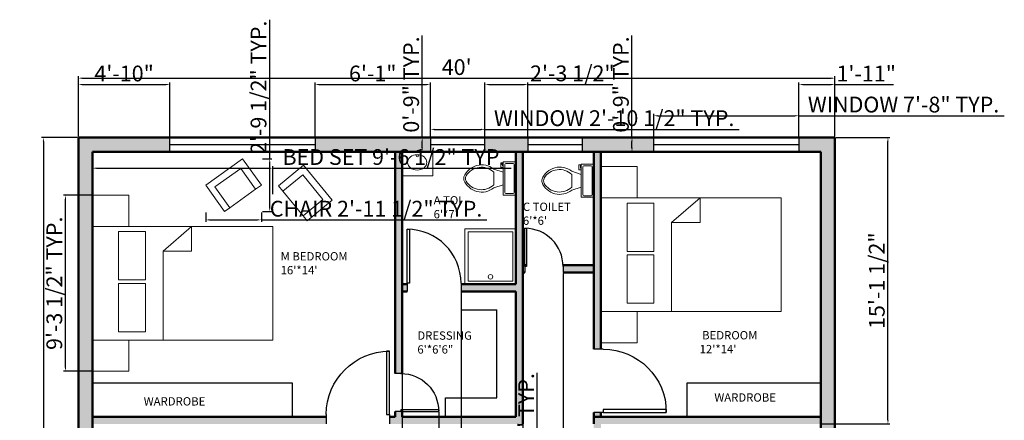
# Model space of a CAD drawing. Units: inches. Extents: x 772 to 1415, y 1573 to 2261.
# Tile 4 of 4: x 790 to 1415, y 2007 to 2261. Entities that reach past the tile are written whole.
import ezdxf

# ---------------------------------------------------------------- set-up
doc = ezdxf.new("R2010")
doc.units = ezdxf.units.IN
for name, color, linetype, lineweight in [('A-ANNO-DIMS', 2, 'Continuous', 18), ('A-ANNO-TEXT', 10, 'Continuous', 25), ('A-AREA-IDEN', 10, 'Continuous', 25), ('A-FLOR-FIXT', 9, 'Continuous', 18), ('A-FURN-FIXD', 210, 'Continuous', 25), ('A-WALL-PATT', 140, 'Continuous', 13), ('DOOR', 52, 'Continuous', 25), ('FUR', 210, 'Continuous', 18), ('WALL', 7, 'Continuous', 50), ('WINDOW', 80, 'Continuous', 25)]:
    doc.layers.add(name, color=color, linetype=linetype, lineweight=lineweight)
doc.styles.get("Standard").update_dxf_attribs({"font": 'arial.ttf'})
doc.dimstyles.new('ISO-25', dxfattribs={"dimtxt": 10, "dimasz": 2.5, "dimexe": 1.25, "dimexo": 0.625, "dimtad": 1, "dimdec": 0, "dimlunit": 4, "dimtxsty": 'Standard', "dimcen": 2.5, "dimadec": 0, "dimazin": 0, "dimtfac": 1, "dimtdec": 0, "dimtmove": 0, "dimatfit": 3, "dimfxl": 1, "dimarcsym": 0})

# ---------------------------------------------------------------- blocks, each defined once
blk = doc.blocks.new('*U2')
for p, q in [((0, 0), (0, -6)), ((40, 0), (40, -6))]:
    blk.add_line(p, q)
blk.add_lwpolyline([(0, 0), (0, 40), (1.75, 40), (1.75, 0)], close=True)
blk.add_arc((0, 0), 40, 0, 90)
blk = doc.blocks.new('*U4')
for p, q in [((9.5, -6), (9.5, -2)), ((-10, -8.5), (-8, -8.5)), ((-10, -9.5), (-10, -8.5)), ((-7, -9.5), (-10, -9.5)), ((-8, -8.5), (-8, -8)), ((-7, -8), (-7, -9.5)), ((-4, -8), (-6, -14)), ((4, -8), (6, -14)), ((4, -14), (-4, -14))]:
    blk.add_line(p, q)
blk.add_lwpolyline([(10.5, -8), (10.5, 0), (-10.5, 0), (-10.5, -8)], close=True)
for points in [[(-9.5, -2), (-9.5, -6)], [(8.5, -1), (-8.5, -1)], [(-8.5, -7), (8.5, -7)]]:
    blk.add_lwpolyline(points)
for centre, radius, start, end in [((-8.62, -1.88), 0.884, 81.8699, 188.1301), ((-8.62, -6.12), 0.884, 171.8699, 278.1301), ((8.62, -1.88), 0.884, 351.8699, 98.1301), ((8.62, -6.12), 0.884, 261.8699, 8.1301), ((3.52, -21.58), 12.17, 141.46911, 247.97143), ((4.2, -21.82), 11.33, 136.36773, 238.94682), ((-3.52, -21.58), 12.17, 292.02843, 38.53071), ((-4.2, -21.82), 11.33, 301.05301, 43.63209), ((0, -27.88), 4, 245.73182, 294.26817), ((0, -29), 4, 254.86053, 285.13947)]:
    blk.add_arc(centre, radius, start, end)
blk = doc.blocks.new('*D9')
at = {"layer": 'A-ANNO-DIMS', "color": 0, "lineweight": -2, "transparency": 16777216}
for p, q in [((827.65, 2186.61), (827.65, 2224.87)), ((1307.65, 2186.61), (1307.65, 2224.87)), ((830.15, 2223.62), (1305.15, 2223.62))]:
    blk.add_line(p, q, dxfattribs=at)
at = {"layer": 'A-ANNO-DIMS', "color": 0, "transparency": 16777216}
for points in [[(830.15, 2224.04), (830.15, 2223.21), (827.65, 2223.62)], [(1305.15, 2224.04), (1305.15, 2223.21), (1307.65, 2223.62)]]:
    blk.add_solid(points, dxfattribs=at)
at = {"layer": 'Defpoints', "color": 0, "transparency": 16777216}
for p in [(1307.65, 2223.62), (827.65, 2185.98), (1307.65, 2185.98)]:
    blk.add_point(p, dxfattribs=at)
at = {"layer": 'A-ANNO-DIMS', "color": 0, "transparency": 16777216, "insert": (1067.65, 2229.36), "char_height": 10, "attachment_point": 5}
blk.add_mtext("40'", dxfattribs=at)
blk = doc.blocks.new('*D10')
at = {"layer": 'A-ANNO-DIMS', "color": 0, "lineweight": -2, "transparency": 16777216}
for p, q in [((827.03, 2185.98), (804.2, 2185.98)), ((805.45, 2183.48), (805.45, 1648.48)), ((827.03, 1645.98), (804.2, 1645.98))]:
    blk.add_line(p, q, dxfattribs=at)
at = {"layer": 'A-ANNO-DIMS', "color": 0, "transparency": 16777216}
for points in [[(805.04, 2183.48), (805.87, 2183.48), (805.45, 2185.98)], [(805.04, 1648.48), (805.87, 1648.48), (805.45, 1645.98)]]:
    blk.add_solid(points, dxfattribs=at)
at = {"layer": 'Defpoints', "color": 0, "transparency": 16777216}
for p in [(827.65, 2185.98), (805.45, 1645.98), (827.65, 1645.98)]:
    blk.add_point(p, dxfattribs=at)
at = {"layer": 'A-ANNO-DIMS', "color": 0, "transparency": 16777216, "insert": (799.74, 1915.98), "char_height": 10, "attachment_point": 5, "rotation": 90}
blk.add_mtext("45'", dxfattribs=at)
blk = doc.blocks.new('BED-DOUBLE-WITH-NIGHTSTANDS')
for p, q in [((62.88, 91.88), (44.81, 76.26)), ((62.88, 76.26), (62.88, 91.88)), ((44.81, 19.73), (44.81, 76.26)), ((44.81, 76.26), (62.88, 76.26))]:
    blk.add_line(p, q)
for points in [[(0, 91.88), (23.11, 91.88), (23.11, 111.61), (0, 111.61)], [(0, 19.73), (114.34, 19.73), (114.34, 91.88), (0, 91.88)], [(16.57, 57.89), (33.66, 57.89), (33.66, 88.54), (16.57, 88.54)], [(16.57, 25.11), (33.66, 25.11), (33.66, 55.76), (16.57, 55.76)], [(0, 0), (23.11, 0), (23.11, 19.73), (0, 19.73)]]:
    blk.add_lwpolyline(points, close=True)
blk = doc.blocks.new('CHAIR-BEDROOM')
for p, q in [((0, 16.64), (23.37, 33.43)), ((23.37, 33.43), (35.32, 16.78)), ((11.95, 0), (0, 16.64)), ((35.32, 16.78), (31.69, 14.18)), ((15.31, 2.41), (11.95, 0))]:
    blk.add_line(p, q)
blk.add_lwpolyline([(15.31, 2.41), (31.69, 14.18), (22.24, 27.34), (5.85, 15.57)], close=True)
blk = doc.blocks.new('WIN-92IN')
blk.add_line((0, 4.5), (92.1, 4.5))
blk.add_lwpolyline([(0, 9), (92.1, 9), (92.1, 0), (0, 0)], close=True)
blk = doc.blocks.new('WIN-35IN')
blk.add_line((0, 4.5), (34.63, 4.5))
blk.add_lwpolyline([(0, 0), (34.63, 0), (34.63, 9), (0, 9)], close=True)
blk = doc.blocks.new('*D21')
at = {"layer": 'A-ANNO-DIMS', "color": 0, "lineweight": -2, "transparency": 16777216}
for p, q in [((836.65, 2150.03), (836.65, 2167.81)), ((950.99, 2150.03), (950.99, 2167.81)), ((839.15, 2166.56), (948.49, 2166.56)), ((950.99, 2166.56), (1102.21, 2166.56))]:
    blk.add_line(p, q, dxfattribs=at)
at = {"layer": 'A-ANNO-DIMS', "color": 0, "transparency": 16777216}
for points in [[(839.15, 2166.97), (839.15, 2166.14), (836.65, 2166.56)], [(948.49, 2166.97), (948.49, 2166.14), (950.99, 2166.56)]]:
    blk.add_solid(points, dxfattribs=at)
at = {"layer": 'Defpoints', "color": 0, "transparency": 16777216}
for p in [(950.99, 2166.56), (836.65, 2149.41), (950.99, 2149.41)]:
    blk.add_point(p, dxfattribs=at)
at = {"layer": 'A-ANNO-DIMS', "color": 0, "transparency": 16777216, "insert": (1027.85, 2172.35), "char_height": 10, "attachment_point": 5}
blk.add_mtext('BED SET 9\'-6 1/2" TYP.', dxfattribs=at)
blk = doc.blocks.new('*D22')
at = {"layer": 'A-ANNO-DIMS', "color": 0, "lineweight": -2, "transparency": 16777216}
for p, q in [((836.03, 2149.41), (818.25, 2149.41)), ((819.5, 2040.29), (819.5, 2146.91)), ((836.03, 2037.79), (818.25, 2037.79))]:
    blk.add_line(p, q, dxfattribs=at)
at = {"layer": 'A-ANNO-DIMS', "color": 0, "transparency": 16777216}
for points in [[(819.08, 2146.91), (819.92, 2146.91), (819.5, 2149.41)], [(819.08, 2040.29), (819.92, 2040.29), (819.5, 2037.79)]]:
    blk.add_solid(points, dxfattribs=at)
at = {"layer": 'Defpoints', "color": 0, "transparency": 16777216}
for p in [(819.5, 2149.41), (836.65, 2149.41), (836.65, 2037.79)]:
    blk.add_point(p, dxfattribs=at)
at = {"layer": 'A-ANNO-DIMS', "color": 0, "transparency": 16777216, "insert": (813.7, 2093.6), "char_height": 10, "attachment_point": 5, "rotation": 90}
blk.add_mtext('9\'-3 1/2" TYP.', dxfattribs=at)
blk = doc.blocks.new('*D23')
at = {"layer": 'A-ANNO-DIMS', "color": 0, "lineweight": -2, "transparency": 16777216}
for p, q in [((908.44, 2138.46), (908.44, 2132.54)), ((943.76, 2138.46), (943.76, 2132.54)), ((910.94, 2133.79), (941.26, 2133.79)), ((943.76, 2133.79), (1086.77, 2133.79))]:
    blk.add_line(p, q, dxfattribs=at)
at = {"layer": 'A-ANNO-DIMS', "color": 0, "transparency": 16777216}
for points in [[(910.94, 2134.21), (910.94, 2133.37), (908.44, 2133.79)], [(941.26, 2134.21), (941.26, 2133.37), (943.76, 2133.79)]]:
    blk.add_solid(points, dxfattribs=at)
at = {"layer": 'Defpoints', "color": 0, "transparency": 16777216}
for p in [(908.44, 2139.09), (943.76, 2139.09), (943.76, 2133.79)]:
    blk.add_point(p, dxfattribs=at)
at = {"layer": 'A-ANNO-DIMS', "color": 0, "transparency": 16777216, "insert": (1016.52, 2139.58), "char_height": 10, "attachment_point": 5}
blk.add_mtext('CHAIR 2\'-11 1/2" TYP.', dxfattribs=at)
blk = doc.blocks.new('*D24')
at = {"layer": 'A-ANNO-DIMS', "color": 0, "lineweight": -2, "transparency": 16777216}
for p, q in [((949.06, 2172.52), (949.06, 2260.69)), ((944.39, 2172.52), (950.31, 2172.52)), ((949.06, 2141.59), (949.06, 2170.02)), ((944.39, 2139.09), (950.31, 2139.09))]:
    blk.add_line(p, q, dxfattribs=at)
at = {"layer": 'A-ANNO-DIMS', "color": 0, "transparency": 16777216}
for points in [[(948.64, 2170.02), (949.48, 2170.02), (949.06, 2172.52)], [(948.64, 2141.59), (949.48, 2141.59), (949.06, 2139.09)]]:
    blk.add_solid(points, dxfattribs=at)
at = {"layer": 'Defpoints', "color": 0, "transparency": 16777216}
for p in [(943.76, 2172.52), (949.06, 2172.52), (943.76, 2139.09)]:
    blk.add_point(p, dxfattribs=at)
at = {"layer": 'A-ANNO-DIMS', "color": 0, "transparency": 16777216, "insert": (943.27, 2217.85), "char_height": 10, "attachment_point": 5, "rotation": 90}
blk.add_mtext('2\'-9 1/2" TYP.', dxfattribs=at)
blk = doc.blocks.new('*D30')
at = {"layer": 'A-ANNO-DIMS', "color": 0, "lineweight": -2, "transparency": 16777216}
for p, q in [((1118.67, 1965.32), (1118.67, 2036.85)), ((1107.43, 1965.32), (1119.92, 1965.32)), ((1118.67, 1944.62), (1118.67, 1962.82)), ((1107.43, 1942.12), (1119.92, 1942.12))]:
    blk.add_line(p, q, dxfattribs=at)
at = {"layer": 'A-ANNO-DIMS', "color": 0, "transparency": 16777216}
for points in [[(1118.25, 1962.82), (1119.09, 1962.82), (1118.67, 1965.32)], [(1118.25, 1944.62), (1119.09, 1944.62), (1118.67, 1942.12)]]:
    blk.add_solid(points, dxfattribs=at)
at = {"layer": 'Defpoints', "color": 0, "transparency": 16777216}
for p in [(1106.81, 1965.32), (1118.67, 1965.32), (1106.81, 1942.12)]:
    blk.add_point(p, dxfattribs=at)
at = {"layer": 'A-ANNO-DIMS', "color": 0, "transparency": 16777216, "insert": (1113.02, 2002.34), "char_height": 10, "attachment_point": 5, "rotation": 90}
blk.add_mtext('1\'-11" TYP.', dxfattribs=at)
blk = doc.blocks.new('*D31')
at = {"layer": 'A-ANNO-DIMS', "color": 0, "lineweight": -2, "transparency": 16777216}
for p, q in [((1192.68, 2186.61), (1192.68, 2201.05)), ((1195.18, 2199.8), (1282.28, 2199.8)), ((1284.78, 2186.61), (1284.78, 2201.05)), ((1284.78, 2199.8), (1415.07, 2199.8))]:
    blk.add_line(p, q, dxfattribs=at)
at = {"layer": 'A-ANNO-DIMS', "color": 0, "transparency": 16777216}
for points in [[(1195.18, 2200.21), (1195.18, 2199.38), (1192.68, 2199.8)], [(1282.28, 2200.21), (1282.28, 2199.38), (1284.78, 2199.8)]]:
    blk.add_solid(points, dxfattribs=at)
at = {"layer": 'Defpoints', "color": 0, "transparency": 16777216}
for p in [(1284.78, 2199.8), (1192.68, 2185.98), (1284.78, 2185.98)]:
    blk.add_point(p, dxfattribs=at)
at = {"layer": 'A-ANNO-DIMS', "color": 0, "transparency": 16777216, "insert": (1351.17, 2205.6), "char_height": 10, "attachment_point": 5}
blk.add_mtext('WINDOW 7\'-8" TYP.', dxfattribs=at)
blk = doc.blocks.new('*D32')
at = {"layer": 'A-ANNO-DIMS', "color": 0, "lineweight": -2, "transparency": 16777216}
for p, q in [((1178.87, 2185.98), (1178.87, 2250.69)), ((1192.06, 2185.98), (1177.62, 2185.98)), ((1178.87, 2179.48), (1178.87, 2183.48)), ((1192.06, 2176.98), (1177.62, 2176.98))]:
    blk.add_line(p, q, dxfattribs=at)
at = {"layer": 'A-ANNO-DIMS', "color": 0, "transparency": 16777216}
for points in [[(1178.45, 2183.48), (1179.28, 2183.48), (1178.87, 2185.98)], [(1178.45, 2179.48), (1179.28, 2179.48), (1178.87, 2176.98)]]:
    blk.add_solid(points, dxfattribs=at)
at = {"layer": 'Defpoints', "color": 0, "transparency": 16777216}
for p in [(1178.87, 2185.98), (1192.68, 2185.98), (1192.68, 2176.98)]:
    blk.add_point(p, dxfattribs=at)
at = {"layer": 'A-ANNO-DIMS', "color": 0, "transparency": 16777216, "insert": (1173.13, 2219.59), "char_height": 10, "attachment_point": 5, "rotation": 90}
blk.add_mtext('0\'-9" TYP.', dxfattribs=at)
blk = doc.blocks.new('*D33')
at = {"layer": 'A-ANNO-DIMS', "color": 0, "lineweight": -2, "transparency": 16777216}
for p, q in [((1050.98, 2186.61), (1050.98, 2192.43)), ((1053.48, 2191.18), (1083.11, 2191.18)), ((1085.61, 2186.61), (1085.61, 2192.43)), ((1085.61, 2191.18), (1246.97, 2191.18))]:
    blk.add_line(p, q, dxfattribs=at)
at = {"layer": 'A-ANNO-DIMS', "color": 0, "transparency": 16777216}
for points in [[(1053.48, 2191.59), (1053.48, 2190.76), (1050.98, 2191.18)], [(1083.11, 2191.59), (1083.11, 2190.76), (1085.61, 2191.18)]]:
    blk.add_solid(points, dxfattribs=at)
at = {"layer": 'Defpoints', "color": 0, "transparency": 16777216}
for p in [(1085.61, 2191.18), (1050.98, 2185.98), (1085.61, 2185.98)]:
    blk.add_point(p, dxfattribs=at)
at = {"layer": 'A-ANNO-DIMS', "color": 0, "transparency": 16777216, "insert": (1167.54, 2196.98), "char_height": 10, "attachment_point": 5}
blk.add_mtext('WINDOW 2\'-10 1/2" TYP.', dxfattribs=at)
blk = doc.blocks.new('*D34')
at = {"layer": 'A-ANNO-DIMS', "color": 0, "lineweight": -2, "transparency": 16777216}
for p, q in [((1045.79, 2185.98), (1045.79, 2250.69)), ((1050.36, 2185.98), (1044.54, 2185.98)), ((1045.79, 2179.48), (1045.79, 2183.48)), ((1050.36, 2176.98), (1044.54, 2176.98))]:
    blk.add_line(p, q, dxfattribs=at)
at = {"layer": 'A-ANNO-DIMS', "color": 0, "transparency": 16777216}
for points in [[(1045.37, 2183.48), (1046.2, 2183.48), (1045.79, 2185.98)], [(1045.37, 2179.48), (1046.2, 2179.48), (1045.79, 2176.98)]]:
    blk.add_solid(points, dxfattribs=at)
at = {"layer": 'Defpoints', "color": 0, "transparency": 16777216}
for p in [(1045.79, 2185.98), (1050.98, 2185.98), (1050.98, 2176.98)]:
    blk.add_point(p, dxfattribs=at)
at = {"layer": 'A-ANNO-DIMS', "color": 0, "transparency": 16777216, "insert": (1040.05, 2219.59), "char_height": 10, "attachment_point": 5, "rotation": 90}
blk.add_mtext('0\'-9" TYP.', dxfattribs=at)
blk = doc.blocks.new('*D47')
at = {"layer": 'A-ANNO-DIMS', "color": 0, "lineweight": -2, "transparency": 16777216}
for p, q in [((1308.28, 2185.98), (1342.5, 2185.98)), ((1341.25, 2006.98), (1341.25, 2183.48)), ((1299.28, 2004.48), (1342.5, 2004.48))]:
    blk.add_line(p, q, dxfattribs=at)
at = {"layer": 'A-ANNO-DIMS', "color": 0, "transparency": 16777216}
for points in [[(1340.83, 2183.48), (1341.67, 2183.48), (1341.25, 2185.98)], [(1340.83, 2006.98), (1341.67, 2006.98), (1341.25, 2004.48)]]:
    blk.add_solid(points, dxfattribs=at)
at = {"layer": 'Defpoints', "color": 0, "transparency": 16777216}
for p in [(1307.65, 2185.98), (1341.25, 2185.98), (1298.65, 2004.48)]:
    blk.add_point(p, dxfattribs=at)
at = {"layer": 'A-ANNO-DIMS', "color": 0, "transparency": 16777216, "insert": (1335.46, 2095.23), "char_height": 10, "attachment_point": 5, "rotation": 90}
blk.add_mtext('15\'-1 1/2"', dxfattribs=at)
blk = doc.blocks.new('*D48')
at = {"layer": 'A-ANNO-DIMS', "color": 0, "lineweight": -2, "transparency": 16777216}
for p, q in [((827.65, 2186.61), (827.65, 2220.83)), ((830.15, 2219.58), (883.22, 2219.58)), ((885.72, 2186.61), (885.72, 2220.83))]:
    blk.add_line(p, q, dxfattribs=at)
at = {"layer": 'A-ANNO-DIMS', "color": 0, "transparency": 16777216}
for points in [[(830.15, 2220), (830.15, 2219.17), (827.65, 2219.58)], [(883.22, 2220), (883.22, 2219.17), (885.72, 2219.58)]]:
    blk.add_solid(points, dxfattribs=at)
at = {"layer": 'Defpoints', "color": 0, "transparency": 16777216}
for p in [(885.72, 2219.58), (827.65, 2185.98), (885.72, 2185.98)]:
    blk.add_point(p, dxfattribs=at)
at = {"layer": 'A-ANNO-DIMS', "color": 0, "transparency": 16777216, "insert": (856.68, 2225.31), "char_height": 10, "attachment_point": 5}
blk.add_mtext('4\'-10"', dxfattribs=at)
blk = doc.blocks.new('*D49')
at = {"layer": 'A-ANNO-DIMS', "color": 0, "lineweight": -2, "transparency": 16777216}
for p, q in [((977.81, 2186.61), (977.81, 2220.83)), ((980.31, 2219.58), (1048.48, 2219.58)), ((1050.98, 2186.61), (1050.98, 2220.83))]:
    blk.add_line(p, q, dxfattribs=at)
at = {"layer": 'A-ANNO-DIMS', "color": 0, "transparency": 16777216}
for points in [[(980.31, 2220), (980.31, 2219.17), (977.81, 2219.58)], [(1048.48, 2220), (1048.48, 2219.17), (1050.98, 2219.58)]]:
    blk.add_solid(points, dxfattribs=at)
at = {"layer": 'Defpoints', "color": 0, "transparency": 16777216}
for p in [(1050.98, 2219.58), (977.81, 2185.98), (1050.98, 2185.98)]:
    blk.add_point(p, dxfattribs=at)
at = {"layer": 'A-ANNO-DIMS', "color": 0, "transparency": 16777216, "insert": (1014.4, 2225.31), "char_height": 10, "attachment_point": 5}
blk.add_mtext('6\'-1"', dxfattribs=at)
blk = doc.blocks.new('*D50')
at = {"layer": 'A-ANNO-DIMS', "color": 0, "lineweight": -2, "transparency": 16777216}
for p, q in [((1085.61, 2186.61), (1085.61, 2220.83)), ((1088.11, 2219.58), (1110.38, 2219.58)), ((1112.88, 2186.61), (1112.88, 2220.83)), ((1112.88, 2219.58), (1166.69, 2219.58))]:
    blk.add_line(p, q, dxfattribs=at)
at = {"layer": 'A-ANNO-DIMS', "color": 0, "transparency": 16777216}
for points in [[(1088.11, 2220), (1088.11, 2219.17), (1085.61, 2219.58)], [(1110.38, 2220), (1110.38, 2219.17), (1112.88, 2219.58)]]:
    blk.add_solid(points, dxfattribs=at)
at = {"layer": 'Defpoints', "color": 0, "transparency": 16777216}
for p in [(1112.88, 2219.58), (1085.61, 2185.98), (1112.88, 2185.98)]:
    blk.add_point(p, dxfattribs=at)
at = {"layer": 'A-ANNO-DIMS', "color": 0, "transparency": 16777216, "insert": (1141.04, 2225.38), "char_height": 10, "attachment_point": 5}
blk.add_mtext('2\'-3 1/2"', dxfattribs=at)
blk = doc.blocks.new('*D51')
at = {"layer": 'A-ANNO-DIMS', "color": 0, "lineweight": -2, "transparency": 16777216}
for p, q in [((1284.78, 2186.61), (1284.78, 2220.83)), ((1287.28, 2219.58), (1305.15, 2219.58)), ((1307.65, 2186.61), (1307.65, 2220.83)), ((1307.65, 2219.58), (1344.81, 2219.58))]:
    blk.add_line(p, q, dxfattribs=at)
at = {"layer": 'A-ANNO-DIMS', "color": 0, "transparency": 16777216}
for points in [[(1287.28, 2220), (1287.28, 2219.17), (1284.78, 2219.58)], [(1305.15, 2220), (1305.15, 2219.17), (1307.65, 2219.58)]]:
    blk.add_solid(points, dxfattribs=at)
at = {"layer": 'Defpoints', "color": 0, "transparency": 16777216}
for p in [(1307.65, 2219.58), (1284.78, 2185.98), (1307.65, 2185.98)]:
    blk.add_point(p, dxfattribs=at)
at = {"layer": 'A-ANNO-DIMS', "color": 0, "transparency": 16777216, "insert": (1327.48, 2225.23), "char_height": 10, "attachment_point": 5}
blk.add_mtext('1\'-11"', dxfattribs=at)
blk = doc.blocks.new('*D61')
at = {"layer": 'A-ANNO-DIMS', "color": 0, "lineweight": -2, "transparency": 16777216}
for p, q in [((1056.25, 2011.79), (1056.25, 1580.94)), ((1033.15, 2008.36), (1033.15, 1580.94)), ((1035.65, 1582.19), (1053.75, 1582.19)), ((1056.25, 1582.19), (1093.41, 1582.19))]:
    blk.add_line(p, q, dxfattribs=at)
at = {"layer": 'A-ANNO-DIMS', "color": 0, "transparency": 16777216}
for points in [[(1035.65, 1582.61), (1035.65, 1581.78), (1033.15, 1582.19)], [(1053.75, 1582.61), (1053.75, 1581.78), (1056.25, 1582.19)]]:
    blk.add_solid(points, dxfattribs=at)
at = {"layer": 'Defpoints', "color": 0, "transparency": 16777216}
for p in [(1056.25, 2012.41), (1033.15, 2008.98), (1056.25, 1582.19)]:
    blk.add_point(p, dxfattribs=at)
at = {"layer": 'A-ANNO-DIMS', "color": 0, "transparency": 16777216, "insert": (1076.08, 1587.84), "char_height": 10, "attachment_point": 5}
blk.add_mtext('1\'-11"', dxfattribs=at)
blk = doc.blocks.new('*D62')
at = {"layer": 'A-ANNO-DIMS', "color": 0, "lineweight": -2, "transparency": 16777216}
for p, q in [((1033.15, 2092.36), (1033.15, 1580.94)), ((1070.44, 2092.36), (1070.44, 1580.94)), ((1035.65, 1582.19), (1067.94, 1582.19)), ((1070.44, 1582.19), (1124.06, 1582.19))]:
    blk.add_line(p, q, dxfattribs=at)
at = {"layer": 'A-ANNO-DIMS', "color": 0, "transparency": 16777216}
for points in [[(1035.65, 1582.61), (1035.65, 1581.78), (1033.15, 1582.19)], [(1067.94, 1582.61), (1067.94, 1581.78), (1070.44, 1582.19)]]:
    blk.add_solid(points, dxfattribs=at)
at = {"layer": 'Defpoints', "color": 0, "transparency": 16777216}
for p in [(1033.15, 2092.98), (1070.44, 2092.98), (1070.44, 1582.19)]:
    blk.add_point(p, dxfattribs=at)
at = {"layer": 'A-ANNO-DIMS', "color": 0, "transparency": 16777216, "insert": (1098.5, 1587.99), "char_height": 10, "attachment_point": 5}
blk.add_mtext('3\'-1 1/2"', dxfattribs=at)
blk = doc.blocks.new('*D63')
at = {"layer": 'A-ANNO-DIMS', "color": 0, "lineweight": -2, "transparency": 16777216}
for p, q in [((1109.65, 2099.86), (1109.65, 1580.94)), ((1135.17, 2099.86), (1135.17, 1580.94)), ((1112.15, 1582.19), (1132.67, 1582.19)), ((1135.17, 1582.19), (1188.98, 1582.19))]:
    blk.add_line(p, q, dxfattribs=at)
at = {"layer": 'A-ANNO-DIMS', "color": 0, "transparency": 16777216}
for points in [[(1112.15, 1582.61), (1112.15, 1581.78), (1109.65, 1582.19)], [(1132.67, 1582.61), (1132.67, 1581.78), (1135.17, 1582.19)]]:
    blk.add_solid(points, dxfattribs=at)
at = {"layer": 'Defpoints', "color": 0, "transparency": 16777216}
for p in [(1109.65, 2100.48), (1135.17, 2100.48), (1135.17, 1582.19)]:
    blk.add_point(p, dxfattribs=at)
at = {"layer": 'A-ANNO-DIMS', "color": 0, "transparency": 16777216, "insert": (1163.33, 1587.99), "char_height": 10, "attachment_point": 5}
blk.add_mtext('2\'-1 1/2"', dxfattribs=at)

msp = doc.modelspace()

# ---------------------------------------------------------------- hatches: boundary and pattern name
at = {"layer": 'A-WALL-PATT'}
h = msp.add_hatch(color=256, dxfattribs=at)
h.dxf.hatch_style = 1
h.paths.add_polyline_path([(885.72, 2185.98), (827.65, 2185.98), (827.65, 1992.85), (836.65, 1992.85), (836.65, 2176.98), (885.72, 2176.98)])
h.paths.add_polyline_path([(1050.98, 2185.98), (977.81, 2185.98), (977.81, 2176.98), (1028.65, 2176.98), (1050.98, 2176.98)])
h.paths.add_polyline_path([(1112.88, 2185.98), (1085.61, 2185.98), (1085.61, 2176.98), (1105.15, 2176.98), (1112.88, 2176.98)])
h.paths.add_polyline_path([(1192.68, 2185.98), (1147.51, 2185.98), (1147.51, 2176.98), (1181.65, 2176.98), (1192.68, 2176.98)])
h.paths.add_polyline_path([(1307.65, 2185.98), (1284.78, 2185.98), (1284.78, 2176.98), (1298.65, 2176.98), (1298.65, 1819.98), (1307.65, 1819.98)])
h.paths.add_polyline_path([(1033.15, 2176.98), (1028.65, 2176.98), (1028.65, 2036.41), (1032.25, 2036.41, -0.009373), (1033.15, 2036.4)])
h.paths.add_polyline_path([(1036.22, 2092.98), (1033.15, 2092.98), (1033.15, 2088.48), (1036.22, 2088.48)])
h.paths.add_polyline_path([(1154.65, 2104.98), (1135.16, 2104.98, -0.008763), (1135.17, 2104.13), (1135.17, 2100.48), (1154.65, 2100.48)])
h.paths.add_polyline_path([(1159.15, 2176.98), (1154.65, 2176.98), (1154.65, 2051.78), (1159.15, 2051.78)])
h.paths.add_polyline_path([(914.37, 1839.72), (927.25, 1839.72), (927.25, 1850.6), (914.37, 1850.6)], flags=9)
h.paths.add_polyline_path([(1081.37, 1890.08), (1108.45, 1890.08), (1108.45, 1909.77), (1081.37, 1909.77)], flags=9)
h.paths.add_polyline_path([(1220.18, 1938.14), (1269.92, 1938.14), (1269.92, 1957.83), (1220.18, 1957.83)], flags=9)
h.paths.add_polyline_path([(1219.66, 2046.23), (1263.24, 2046.23), (1263.24, 2065.92), (1219.66, 2065.92)], flags=9)
h.paths.add_polyline_path([(1107.96, 2127.66), (1143.78, 2127.66), (1143.78, 2147.35), (1107.96, 2147.35)], flags=9)
h.paths.add_polyline_path([(1040.84, 2046.02), (1081.99, 2046.02), (1081.99, 2065.72), (1040.84, 2065.72)], flags=9)
h.paths.add_polyline_path([(1051.44, 2131.75), (1073.61, 2131.75), (1073.61, 2151.44), (1051.44, 2151.44)], flags=9)
h.paths.add_polyline_path([(953.87, 2096.26), (1003.05, 2096.26), (1003.05, 2115.95), (953.87, 2115.95)], flags=9)
h = msp.add_hatch(color=256, dxfattribs=at)
h.dxf.hatch_style = 1
h.paths.add_polyline_path([(1109.65, 2176.98), (1105.15, 2176.98), (1105.15, 2092.98), (1072.93, 2092.98), (1070.44, 2092.98), (1070.44, 2088.48), (1105.15, 2088.48), (1105.15, 2008.98), (1093.16, 2008.98), (1033.15, 2008.98), (1033.15, 2012.41), (1032.25, 2012.41), (1028.65, 2012.41), (1028.65, 2008.98), (1024.95, 2008.98), (1024.95, 2004.48), (1033.15, 2004.48), (1109.65, 2004.48), (1109.65, 2008.98), (1109.65, 2088.48)])
h.paths.add_polyline_path([(1159.15, 1958.53), (1154.65, 1958.53), (1154.65, 1819.98), (1185.12, 1819.98), (1185.12, 1828.98), (1159.15, 1828.98)])
h.paths.add_polyline_path([(1298.65, 1828.98), (1273.39, 1828.98), (1273.39, 1819.98), (1298.65, 1819.98)])
h.paths.add_polyline_path([(1107.96, 2127.66), (1143.78, 2127.66), (1143.78, 2147.35), (1107.96, 2147.35)], flags=9)
h = msp.add_hatch(color=256, dxfattribs=at)
h.dxf.hatch_style = 1
h.paths.add_polyline_path([(836.65, 1835.78), (827.65, 1835.78), (827.65, 1770.04), (833.65, 1770.04), (836.65, 1770.04)])
h.paths.add_polyline_path([(1154.65, 1824.48), (938.65, 1824.48), (836.65, 1824.48), (836.65, 1819.98), (980.65, 1819.98), (1154.65, 1819.98)])
h.paths.add_polyline_path([(836.65, 1962.89), (827.65, 1962.89), (827.65, 1865.74), (836.65, 1865.74)])
h.paths.add_polyline_path([(913.15, 1980.86), (910.62, 1980.86, -0.029352), (908.65, 1980.98), (908.65, 1968.98), (900.27, 1968.98), (855.22, 1968.98), (855.22, 1964.48), (913.15, 1964.48)])
h.paths.add_polyline_path([(855.22, 1968.98), (836.65, 1968.98), (836.65, 1964.48), (855.22, 1964.48)])
h.paths.add_polyline_path([(984.95, 2008.98), (836.65, 2008.98), (836.65, 2004.48), (908.65, 2004.48), (984.95, 2004.48)])
h.paths.add_polyline_path([(1298.65, 2008.98), (1171.7, 2008.98), (1154.65, 2008.98), (1154.65, 2004.48), (1298.65, 2004.48)])
h.paths.add_polyline_path([(1159.15, 2011.78), (1154.65, 2011.78), (1154.65, 2008.98), (1159.15, 2008.98)])
h.paths.add_polyline_path([(1159.15, 2004.48), (1154.65, 2004.48), (1154.65, 1998.53), (1159.15, 1998.53)])

# ---------------------------------------------------------------- linework, layer by layer
at = {"layer": 'A-FLOR-FIXT'}
for points in [[(1033.15, 2176.98), (1052.44, 2176.98), (1052.44, 2161.8), (1033.15, 2161.8)], [(1072.93, 2092.98), (1105.15, 2092.98), (1105.15, 2128.14), (1072.93, 2128.14)], [(1074.89, 2094.94), (1103.19, 2094.94), (1103.19, 2126.18), (1074.89, 2126.18)]]:
    msp.add_lwpolyline(points, close=True, dxfattribs=at)
for centre, radius in [((1042.64, 2174.41), 0.712), ((1089.1, 2097.67), 1.44)]:
    msp.add_circle(centre, radius, dxfattribs=at)
msp.add_ellipse((1042.64, 2170.25), major_axis=(6.09, 0), ratio=0.8, dxfattribs=at)
at = {"layer": 'A-FURN-FIXD'}
for p, q in [((1070.44, 2088.48), (1070.44, 2076.85)), ((1070.44, 2076.85), (1093.16, 2076.85)), ((1093.16, 2021.06), (1093.16, 2076.85)), ((1213.6, 2030.33), (1213.6, 2008.98)), ((1060.62, 2008.98), (1060.62, 2021.06)), ((1060.62, 2021.06), (1093.16, 2021.06)), ((1105.15, 2008.98), (1093.16, 2008.98))]:
    msp.add_line(p, q, dxfattribs=at)
msp.add_lwpolyline([(836.65, 2008.98), (963.61, 2008.98), (963.61, 2030.33), (836.65, 2030.33)], close=True, dxfattribs=at)
msp.add_lwpolyline([(1171.7, 2008.98), (1298.65, 2008.98), (1298.65, 2030.33), (1213.6, 2030.33)], dxfattribs=at)
at = {"layer": 'WALL'}
for p, q in [((827.65, 2185.98), (1307.65, 2185.98)), ((827.65, 1770.04), (827.65, 2185.98)), ((1307.65, 2185.98), (1307.65, 1819.98)), ((836.65, 2176.98), (1298.65, 2176.98)), ((836.65, 2176.98), (1028.65, 2176.98)), ((836.65, 1768.29), (836.65, 2176.98)), ((1028.65, 2176.98), (1028.65, 2036.41)), ((1033.15, 2176.98), (1033.15, 2036.4)), ((1033.15, 2176.98), (1105.15, 2176.98)), ((1105.15, 2176.98), (1105.15, 2092.98)), ((1109.65, 2176.98), (1109.65, 2088.48)), ((1109.65, 2176.98), (1181.65, 2176.98)), ((1298.65, 2176.98), (1154.65, 2176.98)), ((1154.65, 2176.98), (1154.65, 2051.78)), ((1159.15, 2176.98), (1159.15, 2051.78)), ((1298.65, 2176.98), (1298.65, 1819.98)), ((1111.92, 2104.98), (1109.65, 2104.98)), ((1110.85, 2100.48), (1109.65, 2100.48)), ((1154.65, 2104.98), (1135.16, 2104.98)), ((1154.65, 2100.48), (1135.17, 2100.48)), ((1036.22, 2092.98), (1033.15, 2092.98)), ((1105.15, 2092.98), (1070.44, 2092.98)), ((1036.22, 2088.48), (1033.15, 2088.48)), ((1105.15, 2088.48), (1070.44, 2088.48)), ((1105.15, 2088.48), (1105.15, 2008.98)), ((1109.65, 2008.98), (1109.65, 2088.48)), ((1028.65, 2012.41), (1028.65, 2008.98)), ((1033.15, 2013.46), (1033.15, 2008.98)), ((1154.65, 2011.78), (1154.65, 2008.98)), ((1159.15, 2011.78), (1159.15, 2008.98)), ((984.95, 2008.98), (836.65, 2008.98)), ((1028.65, 2008.98), (1024.95, 2008.98)), ((1033.15, 2008.98), (1105.15, 2008.98)), ((1109.65, 2008.98), (1109.65, 2004.48)), ((1154.65, 2008.98), (1298.65, 2008.98)), ((1154.65, 2008.98), (1154.65, 2004.48))]:
    msp.add_line(p, q, dxfattribs=at)

# ---------------------------------------------------------------- block references
at = {"layer": 'A-FLOR-FIXT', "rotation": 270}
for p in [(1105.15, 2160.04), (1154.65, 2158.59)]:
    msp.add_blockref('*U4', p, dxfattribs=at)
at = {"layer": 'DOOR'}
for p, xscale, yscale, zscale in [((1036.22, 2093.62), 0.855483859173754, 0.855483859173754, 0.855483859173754), ((1110.85, 2104.13), 0.6079577232164337, 0.6079577232164337, 0.6079577232164337)]:
    msp.add_blockref('*U2', p, dxfattribs=dict(at, xscale=xscale, yscale=yscale, zscale=zscale))
at = {"layer": 'DOOR', "xscale": -1}
msp.add_blockref('*U2', (1024.95, 2010.48), dxfattribs=at)
at = {"layer": 'DOOR', "xscale": -1, "rotation": 270}
msp.add_blockref('*U2', (1160.65, 2011.78), dxfattribs=at)
at = {"layer": 'DOOR', "xscale": -0.6000584940735214, "yscale": 0.6000584940735214, "zscale": 0.6000584940735214, "rotation": 270}
msp.add_blockref('*U2', (1032.25, 2012.41), dxfattribs=at)
at = {"layer": 'FUR'}
for name, p in [('CHAIR-BEDROOM', (908.44, 2139.09)), ('BED-DOUBLE-WITH-NIGHTSTANDS', (1159.15, 2055.94)), ('BED-DOUBLE-WITH-NIGHTSTANDS', (836.65, 2037.79))]:
    msp.add_blockref(name, p, dxfattribs=at)
at = {"layer": 'FUR', "extrusion": (0, 0, -1), "zscale": -1, "rotation": 14.93987707136356}
msp.add_blockref('CHAIR-BEDROOM', (-984.41, 2130.12), dxfattribs=at)
at = {"layer": 'WINDOW'}
for name, p in [('WIN-92IN', (885.72, 2176.98)), ('WIN-35IN', (1050.98, 2176.98)), ('WIN-35IN', (1112.88, 2176.98)), ('WIN-92IN', (1192.68, 2176.98))]:
    msp.add_blockref(name, p, dxfattribs=at)

# ---------------------------------------------------------------- texts
at = {"layer": 'A-ANNO-TEXT', "char_height": 5.277, "attachment_point": 1}
for insert in [(1231.1, 2023.83), (869.11, 2021.38)]:
    msp.add_mtext_dynamic_manual_height_columns('WARDROBE', width=83.1931, gutter_width=26.39, heights=[0], dxfattribs=dict(at, insert=insert))
at = {"layer": 'A-AREA-IDEN', "char_height": 5.277, "attachment_point": 1}
for s, insert in [("A TOI\\P6'*7'", (1053.04, 2148.82)), ("C TOILET\\P6'*6'", (1109.65, 2144.72)), ("M BEDROOM\\P16'*14'", (955.99, 2113.33)), ('DRESSING\\P6\'*6\'6"', (1042.73, 2063.09)), (" BEDROOM\\P12'*14'", (1221.78, 2063.3))]:
    msp.add_mtext_dynamic_manual_height_columns(s, width=83.1931, gutter_width=26.39, heights=[0], dxfattribs=dict(at, insert=insert))

# ---------------------------------------------------------------- dimensions: what is measured, and where the dimension line sits
at = {"layer": 'A-ANNO-DIMS'}
for base, p1, p2, picture, middle in [((949.06, 2172.52), (943.76, 2139.09), (943.76, 2172.52), '*D24', (943.27, 2217.85)), ((1045.79, 2185.98), (1050.98, 2176.98), (1050.98, 2185.98), '*D34', (1040.05, 2219.59)), ((1178.87, 2185.98), (1192.68, 2176.98), (1192.68, 2185.98), '*D32', (1173.13, 2219.59)), ((819.5, 2149.41), (836.65, 2037.79), (836.65, 2149.41), '*D22', (813.7, 2093.6)), ((1118.67, 1965.32), (1106.81, 1942.12), (1106.81, 1965.32), '*D30', (1113.02, 2002.34))]:
    dim = msp.add_linear_dim(base=base, p1=p1, p2=p2, angle=90, text='<> TYP.', dimstyle='ISO-25', override={"dimdec": 1, "dimlfac": 1, "dimrnd": 0, "dimzin": 1, "dimdsep": 46, "dimlunit": 4, "dimfrac": 2}, dxfattribs=at)
    dim.commit()
    dim.dimension.update_dxf_attribs({"geometry": picture, "text_midpoint": middle})
for base, p1, p2, override, picture, middle in [((1112.88, 2219.58), (1085.61, 2185.98), (1112.88, 2185.98), {"dimdec": 1, "dimlfac": 1, "dimrnd": 0, "dimzin": 1, "dimdsep": 46, "dimlunit": 4, "dimfrac": 2}, '*D50', (1141.04, 2225.38)), ((1307.65, 2223.62), (827.65, 2185.98), (1307.65, 2185.98), {"dimclrd": 0, "dimclre": 0, "dimclrt": 0}, '*D9', (1067.65, 2229.36)), ((885.72, 2219.58), (827.65, 2185.98), (885.72, 2185.98), {"dimdec": 1, "dimlfac": 1, "dimrnd": 0, "dimzin": 1, "dimdsep": 46, "dimlunit": 4, "dimfrac": 2}, '*D48', (856.68, 2225.31)), ((1050.98, 2219.58), (977.81, 2185.98), (1050.98, 2185.98), {"dimdec": 1, "dimlfac": 1, "dimrnd": 0, "dimzin": 1, "dimdsep": 46, "dimlunit": 4, "dimfrac": 2}, '*D49', (1014.4, 2225.31)), ((1307.65, 2219.58), (1284.78, 2185.98), (1307.65, 2185.98), {"dimdec": 1, "dimlfac": 1, "dimrnd": 0, "dimzin": 1, "dimdsep": 46, "dimlunit": 4, "dimfrac": 2}, '*D51', (1327.48, 2225.23)), ((1135.17, 1582.19), (1109.65, 2100.48), (1135.17, 2100.48), {"dimdec": 1, "dimlfac": 1, "dimrnd": 0, "dimzin": 1, "dimdsep": 46, "dimlunit": 4, "dimfrac": 2}, '*D63', (1163.33, 1587.99)), ((1070.44, 1582.19), (1033.15, 2092.98), (1070.44, 2092.98), {"dimdec": 1, "dimlfac": 1, "dimrnd": 0, "dimzin": 1, "dimdsep": 46, "dimlunit": 4, "dimfrac": 2}, '*D62', (1098.5, 1587.99)), ((1056.25, 1582.19), (1033.15, 2008.98), (1056.25, 2012.41), {"dimdec": 1, "dimlfac": 1, "dimrnd": 0, "dimzin": 1, "dimdsep": 46, "dimlunit": 4, "dimfrac": 2}, '*D61', (1076.08, 1587.84))]:
    dim = msp.add_linear_dim(base=base, p1=p1, p2=p2, dimstyle='ISO-25', override=override, dxfattribs=at)
    dim.commit()
    dim.dimension.update_dxf_attribs({"geometry": picture, "text_midpoint": middle})
for base, p1, p2, text, picture, middle in [((1085.61, 2191.18), (1050.98, 2185.98), (1085.61, 2185.98), 'WINDOW <> TYP.', '*D33', (1167.54, 2196.98)), ((1284.78, 2199.8), (1192.68, 2185.98), (1284.78, 2185.98), 'WINDOW <> TYP.', '*D31', (1351.17, 2205.6)), ((950.99, 2166.56), (836.65, 2149.41), (950.99, 2149.41), 'BED SET <> TYP.', '*D21', (1027.85, 2172.35)), ((943.76, 2133.79), (908.44, 2139.09), (943.76, 2139.09), 'CHAIR <> TYP.', '*D23', (1016.52, 2139.58))]:
    dim = msp.add_linear_dim(base=base, p1=p1, p2=p2, text=text, dimstyle='ISO-25', override={"dimdec": 1, "dimlfac": 1, "dimrnd": 0, "dimzin": 1, "dimdsep": 46, "dimlunit": 4, "dimfrac": 2}, dxfattribs=at)
    dim.commit()
    dim.dimension.update_dxf_attribs({"geometry": picture, "text_midpoint": middle})
for base, p1, p2, override, picture, middle in [((805.45, 1645.98), (827.65, 2185.98), (827.65, 1645.98), {"dimclrd": 0, "dimclre": 0, "dimclrt": 0}, '*D10', (799.74, 1915.98)), ((1341.25, 2185.98), (1298.65, 2004.48), (1307.65, 2185.98), {"dimdec": 1, "dimlfac": 1, "dimrnd": 0, "dimzin": 1, "dimdsep": 46, "dimlunit": 4, "dimfrac": 2}, '*D47', (1335.46, 2095.23))]:
    dim = msp.add_linear_dim(base=base, p1=p1, p2=p2, angle=90, dimstyle='ISO-25', override=override, dxfattribs=at)
    dim.commit()
    dim.dimension.update_dxf_attribs({"geometry": picture, "text_midpoint": middle})

doc.saveas('drawing.dxf')
